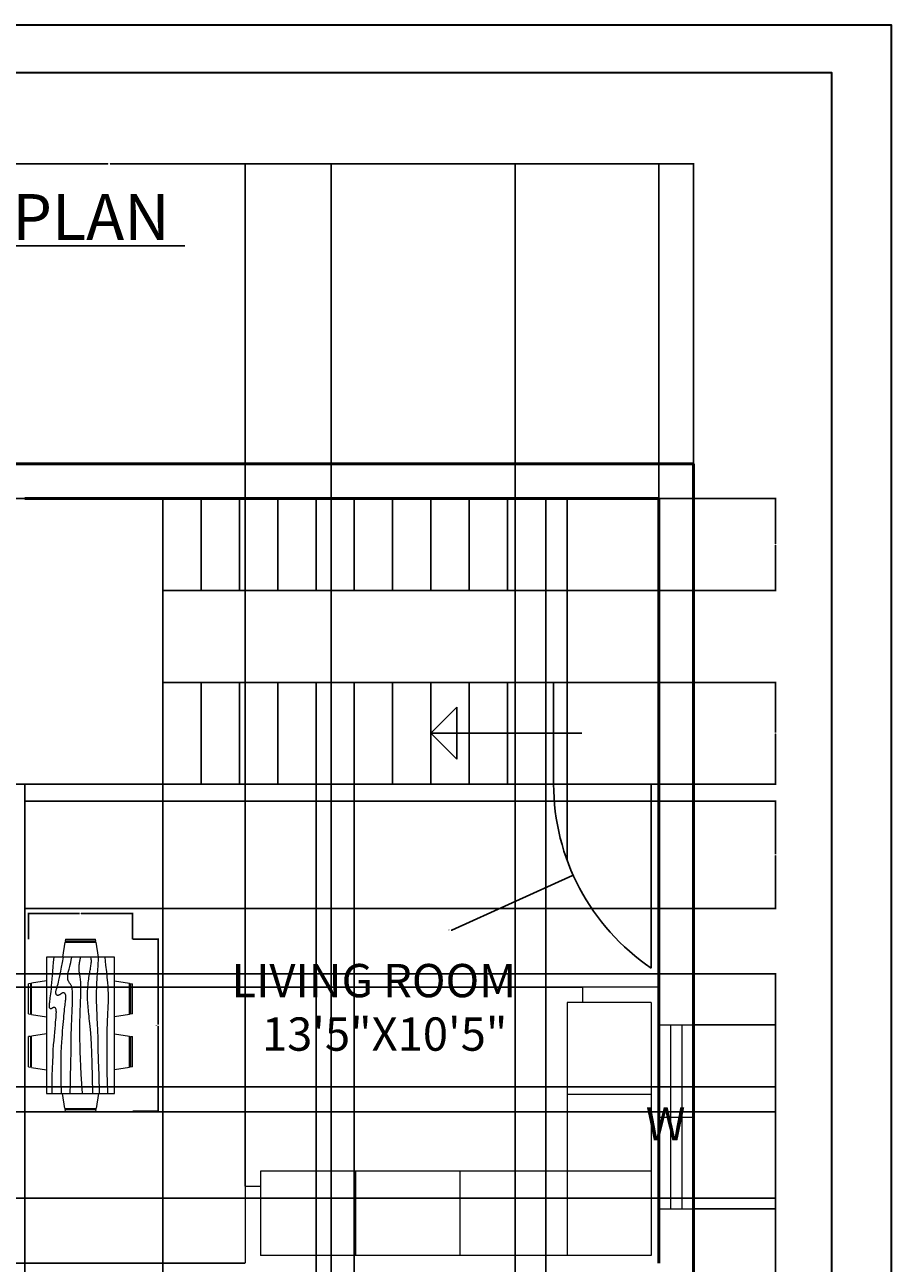
# Model space of a CAD drawing. Units: inches. Extents: x 1804 to 2221, y 1838 to 2403.
# Tile 3 of 3: x 1995 to 2221, y 2079 to 2403. Entities that reach past the tile are written whole.
import ezdxf

# ---------------------------------------------------------------- set-up
doc = ezdxf.new("R2010")
doc.units = ezdxf.units.IN
for name, color, linetype, lineweight in [('A-ANNO-DIMS', 2, 'Continuous', 18), ('A-ANNO-TEXT', 7, 'Continuous', 25), ('A-ANNO-TTLB', 7, 'Continuous', 35), ('A-AREA-IDEN', 7, 'Continuous', 25), ('A-DOOR', 3, 'Continuous', 25), ('A-FLOR-STRS', 7, 'Continuous', 25), ('A-FURN', 8, 'Continuous', 18), ('A-GLAZ', 4, 'Continuous', 18), ('A-WALL', 7, 'Continuous', 50)]:
    doc.layers.add(name, color=color, linetype=linetype, lineweight=lineweight)
doc.styles.get("Standard").update_dxf_attribs({"font": 'arial.ttf'})
doc.dimstyles.get("Standard").update_dxf_attribs({"dimtxt": 0.18, "dimasz": 0.18, "dimexe": 0.18, "dimexo": 0.0625, "dimgap": 0.09, "dimtad": 0, "dimtih": 1, "dimtoh": 1, "dimdec": 4, "dimzin": 0, "dimdsep": 46, "dimtxsty": 'Standard', "dimcen": 0.09, "dimadec": 0, "dimazin": 0, "dimtfac": 1, "dimtdec": 4, "dimtofl": 0, "dimtmove": 0, "dimatfit": 3, "dimfxl": 1, "dimtolj": 1, "dimtzin": 0, "dimarcsym": 0})

# ---------------------------------------------------------------- blocks, each defined once
blk = doc.blocks.new('Dining Set - 36 x 72 in.')
for p, q in [((-22, 27.5), (-22.1562, 26.50042)), ((-5.8416, 26.5), (-22.1534, 26.5)), ((-22, 27.5), (-6, 27.5)), ((-5.8437, 26.49966), (-6, 27.5)), ((6, 27.5), (5.8438, 26.50042)), ((22.1584, 26.5), (5.8466, 26.5)), ((6, 27.5), (22, 27.5)), ((22.1563, 26.49966), (22, 27.5)), ((-22.2343, 26.00059), (-23.4847, 17.99762)), ((-22.2304, 26), (-5.7608, 26)), ((-4.5152, 17.99762), (-5.7655, 25.99926)), ((5.7657, 26.00059), (4.5153, 17.99762)), ((5.7696, 26), (22.2392, 26)), ((23.4848, 17.99762), (22.2345, 25.99926)), ((36, 18), (-36, 18)), ((-36, 18), (-36, -18)), ((36, -18), (36, 18)), ((-45.5, 8), (-44.5004, 8.15617)), ((-45.5, 8), (-45.5, -8)), ((-44.5, -8.15843), (-44.5, 8.15338)), ((-44.0006, 8.23428), (-35.9976, 9.48474)), ((-44, 8.23041), (-44, -8.23915)), ((44.0006, 8.23428), (35.9976, 9.48474)), ((44, 8.23041), (44, -8.23915)), ((44.5, -8.15843), (44.5, 8.15338)), ((45.5, 8), (44.5005, 8.15617)), ((45.5, 8), (45.5, -8)), ((-44.4997, -8.15631), (-45.5, -8)), ((-35.9976, -9.48476), (-43.9993, -8.2345)), ((35.9976, -9.48476), (43.9993, -8.2345)), ((44.4997, -8.15631), (45.5, -8)), ((-36, -18), (36, -18)), ((-22.2343, -26.0006), (-23.4847, -17.99762)), ((-4.5152, -17.99762), (-5.7655, -25.99928)), ((5.7657, -26.0006), (4.5153, -17.99762)), ((23.4848, -17.99762), (22.2345, -25.99928)), ((-22.2304, -26), (-5.7608, -26)), ((5.7696, -26), (22.2392, -26)), ((-22, -27.5), (-22.1562, -26.50044)), ((-5.8416, -26.5), (-22.1534, -26.5)), ((-22, -27.5), (-6, -27.5)), ((-5.8437, -26.49967), (-6, -27.5)), ((6, -27.5), (5.8438, -26.50044)), ((22.1584, -26.5), (5.8466, -26.5)), ((6, -27.5), (22, -27.5)), ((22.1563, -26.49967), (22, -27.5))]:
    blk.add_line(p, q)
for points in [[(-36, 15), (-31.1772, 14.97754), (-26.8079, 14.91406), (-22.8538, 14.81543), (-19.276, 14.6875), (-16.0362, 14.53613), (-13.0957, 14.36718), (-10.4159, 14.18652), (-7.9583, 14), (-5.6904, 13.81315), (-3.6035, 13.63021), (-1.6954, 13.45508), (0.0365, 13.29166), (1.5945, 13.14388), (2.9811, 13.01562), (4.1988, 12.9108), (5.25, 12.83333), (6.1393, 12.78613), (6.8802, 12.76823), (7.4883, 12.77767), (7.9792, 12.8125), (8.3685, 12.87077), (8.6719, 12.95052), (8.9049, 13.0498), (9.0833, 13.16666), (9.2205, 13.29899), (9.3216, 13.44401), (9.3895, 13.59879), (9.4271, 13.76041), (9.4373, 13.92594), (9.4232, 14.09245), (9.3875, 14.257), (9.3333, 14.41666), (9.2638, 14.56917), (9.1836, 14.71484), (9.0975, 14.85465), (9.0104, 14.98958), (8.9272, 15.1206), (8.8529, 15.2487), (8.7922, 15.37483), (8.75, 15.5), (8.7305, 15.62467), (8.7344, 15.74739), (8.7617, 15.86621), (8.8125, 15.97916), (8.8867, 16.08431), (8.9844, 16.17968), (9.1055, 16.26334), (9.25, 16.33333), (9.4189, 16.38802), (9.6172, 16.42708), (9.8506, 16.45052), (10.125, 16.45833), (10.4463, 16.45052), (10.8203, 16.42708), (11.2529, 16.38802), (11.75, 16.33333), (12.3184, 16.26318), (12.9694, 16.17838), (13.7151, 16.07991), (14.5677, 15.96875), (15.5395, 15.84586), (16.6426, 15.71224), (17.8893, 15.56884), (19.2917, 15.41666), (20.859, 15.25667), (22.5879, 15.08984), (24.4721, 14.91715), (26.5052, 14.73958), (28.6809, 14.5581), (30.9929, 14.3737), (33.4347, 14.18733), (36, 14)], [(-36, 10), (-28.9766, 10.14274), (-23.1725, 10.20442), (-18.4241, 10.19775), (-14.5677, 10.13541), (-11.4399, 10.03011), (-8.877, 9.89453), (-6.7154, 9.74137), (-4.7917, 9.58333), (-2.9698, 9.43082), (-1.2246, 9.28515), (0.4415, 9.14534), (2.026, 9.01041), (3.5266, 8.87939), (4.9408, 8.7513), (6.266, 8.62516), (7.5, 8.5), (8.6411, 8.37549), (9.6914, 8.2539), (10.6538, 8.13818), (11.5312, 8.03125), (12.3267, 7.93603), (13.043, 7.85547), (13.6831, 7.79248), (14.25, 7.75), (14.7471, 7.7303), (15.1797, 7.73307), (15.5537, 7.75732), (15.875, 7.80208), (16.1494, 7.86637), (16.3828, 7.94922), (16.5811, 8.04964), (16.75, 8.16666), (16.8944, 8.29915), (17.0143, 8.44531), (17.1089, 8.60319), (17.1771, 8.77083), (17.218, 8.94629), (17.2305, 9.1276), (17.2137, 9.31282), (17.1667, 9.5), (17.0895, 9.6875), (16.987, 9.875), (16.8649, 10.0625), (16.7292, 10.25), (16.5856, 10.4375), (16.4401, 10.625), (16.2985, 10.8125), (16.1667, 11), (16.05, 11.18733), (15.9518, 11.3737), (15.8752, 11.5581), (15.8229, 11.73958), (15.798, 11.91715), (15.8034, 12.08984), (15.842, 12.25667), (15.9167, 12.41666), (16.0295, 12.56836), (16.1784, 12.70833), (16.3605, 12.83268), (16.5729, 12.9375), (16.8127, 13.01888), (17.0768, 13.07291), (17.3625, 13.0957), (17.6667, 13.08333), (17.9894, 13.03312), (18.3418, 12.94726), (18.7382, 12.82918), (19.1927, 12.68229), (19.7195, 12.51001), (20.3327, 12.31575), (21.0465, 12.10294), (21.875, 11.875), (22.8357, 11.63354), (23.959, 11.37304), (25.2786, 11.08618), (26.8282, 10.76562), (28.6414, 10.40405), (30.752, 9.99414), (33.1936, 9.52856), (36, 9)], [(-36, 5.5), (-30.7157, 5.3348), (-26.069, 5.20963), (-21.9946, 5.11767), (-18.4271, 5.05208), (-15.3009, 5.00602), (-12.5508, 4.97265), (-10.1112, 4.94515), (-7.9167, 4.91666), (-5.909, 4.88167), (-4.0586, 4.83984), (-2.3429, 4.79215), (-0.7396, 4.73958), (0.7739, 4.6831), (2.22, 4.6237), (3.6213, 4.56233), (5, 4.5), (6.373, 4.43782), (7.7344, 4.3776), (9.0723, 4.32129), (10.375, 4.27083), (11.6309, 4.22819), (12.8281, 4.19531), (13.9551, 4.17415), (15, 4.16666), (15.954, 4.17448), (16.819, 4.19791), (17.6001, 4.23698), (18.3021, 4.29166), (18.9299, 4.36198), (19.4883, 4.44791), (19.9823, 4.54948), (20.4167, 4.66666), (20.7969, 4.79899), (21.1302, 4.94401), (21.4245, 5.09879), (21.6875, 5.26041), (21.9271, 5.42594), (22.1511, 5.59245), (22.3672, 5.757), (22.5834, 5.91666), (22.8065, 6.06868), (23.0404, 6.21093), (23.2879, 6.34147), (23.5521, 6.45833), (23.8358, 6.55957), (24.142, 6.64323), (24.4735, 6.70735), (24.8334, 6.75), (25.2235, 6.76969), (25.642, 6.76692), (26.0858, 6.74267), (26.5521, 6.69791), (27.0379, 6.63362), (27.5404, 6.55078), (28.0565, 6.45036), (28.5834, 6.33333), (29.1242, 6.19987), (29.7071, 6.04687), (30.3661, 5.87044), (31.1354, 5.66666), (32.0493, 5.43164), (33.142, 5.16146), (34.4475, 4.85221), (36, 4.5)], [(-36, -1), (-30.7915, -0.6591), (-26.0195, -0.38216), (-21.6519, -0.16284), (-17.6563, 0.00521), (-14.0005, 0.12833), (-10.6523, 0.21289), (-7.5796, 0.26522), (-4.75, 0.29166), (-2.134, 0.29793), (0.2878, 0.28711), (2.5317, 0.26163), (4.6146, 0.22396), (6.5529, 0.17651), (8.3633, 0.12174), (10.0623, 0.06209), (11.6667, 0), (13.1899, -0.06201), (14.6341, -0.1211), (15.9982, -0.17432), (17.2813, -0.21875), (18.4823, -0.25147), (19.6003, -0.26953), (20.6343, -0.27002), (21.5834, -0.25), (22.4481, -0.20768), (23.2357, -0.14584), (23.9549, -0.06836), (24.6146, 0.02083), (25.2235, 0.11784), (25.7904, 0.21875), (26.3241, 0.31966), (26.8334, 0.41666), (27.3265, 0.50618), (27.8099, 0.58593), (28.2894, 0.65397), (28.7709, 0.70833), (29.2601, 0.74707), (29.763, 0.76823), (30.2855, 0.76985), (30.8334, 0.75), (31.4088, 0.70784), (31.9994, 0.64713), (32.589, 0.57275), (33.1615, 0.48958), (33.7008, 0.4025), (34.1908, 0.3164), (34.6153, 0.23616), (34.9584, 0.16666), (35.2099, 0.11165), (35.3848, 0.07031), (35.504, 0.04069), (35.5886, 0.02083), (35.6594, 0.00879), (35.7377, 0.0026), (35.8442, 0.00032), (36, 0)], [(-36, -6.5), (-27.1843, -6.31267), (-20.084, -6.1263), (-14.469, -5.9419), (-10.1094, -5.76042), (-6.7752, -5.58285), (-4.2363, -5.41016), (-2.2629, -5.24333), (-0.625, -5.08334), (0.8708, -4.93099), (2.2715, -4.78646), (3.5872, -4.64974), (4.8281, -4.52084), (6.0046, -4.39974), (7.127, -4.28646), (8.2053, -4.18099), (9.25, -4.08334), (10.2705, -3.99382), (11.2734, -3.91407), (12.2647, -3.84603), (13.25, -3.79167), (14.2354, -3.75293), (15.2266, -3.73177), (16.2295, -3.73015), (17.25, -3.75), (18.2912, -3.79248), (19.3451, -3.85547), (20.4009, -3.93604), (21.4479, -4.03125), (22.4754, -4.13819), (23.4727, -4.25391), (24.4289, -4.37549), (25.3334, -4.5), (26.1785, -4.62492), (26.9694, -4.74935), (27.7145, -4.87281), (28.4219, -4.99479), (29.1, -5.11483), (29.7572, -5.23242), (30.4016, -5.34709), (31.0417, -5.45834), (31.6837, -5.56437), (32.3262, -5.65821), (32.9658, -5.73153), (33.599, -5.77604), (34.2224, -5.78345), (34.8327, -5.74545), (35.4264, -5.65373), (36, -5.5)], [(-36, -10), (-26.4022, -9.81299), (-18.4675, -9.62891), (-11.9839, -9.45069), (-6.7396, -9.28125), (-2.5226, -9.12354), (0.8789, -8.98047), (3.6769, -8.85498), (6.0833, -8.75), (8.2767, -8.66765), (10.3021, -8.60677), (12.1712, -8.56543), (13.8958, -8.54167), (15.4876, -8.53353), (16.9583, -8.53907), (18.3197, -8.55632), (19.5834, -8.58334), (20.7616, -8.61841), (21.8685, -8.66081), (22.9188, -8.71004), (23.9271, -8.76563), (24.9081, -8.82707), (25.8763, -8.89388), (26.8465, -8.96558), (27.8334, -9.04167), (28.8474, -9.12118), (29.8828, -9.20117), (30.93, -9.27824), (31.9792, -9.34896), (33.0205, -9.40991), (34.0443, -9.45768), (35.0407, -9.48885), (36, -9.5)], [(-36, -14.5), (-30.0881, -14.33513), (-25.0332, -14.21224), (-20.7312, -14.12647), (-17.0781, -14.07292), (-13.97, -14.04671), (-11.3027, -14.04297), (-8.9724, -14.05681), (-6.875, -14.08334), (-4.9224, -14.11833), (-3.0905, -14.16016), (-1.3709, -14.20785), (0.2448, -14.26042), (1.7647, -14.3169), (3.1973, -14.3763), (4.5507, -14.43767), (5.8333, -14.5), (7.0554, -14.5621), (8.235, -14.62175), (9.3922, -14.67652), (10.5469, -14.72396), (11.7192, -14.76164), (12.929, -14.78711), (14.1965, -14.79794), (15.5417, -14.79167), (16.9933, -14.76424), (18.6152, -14.70508), (20.4804, -14.60197), (22.6615, -14.44271), (25.2312, -14.21509), (28.2624, -13.9069), (31.8277, -13.50594), (36, -13)]]:
    blk.add_lwpolyline(points)
blk = doc.blocks.new('*D18')
at = {"layer": 'A-ANNO-DIMS', "color": 0, "lineweight": -2, "transparency": 16777216}
for p, q in [((2022.76, 2163.97), (2029.61, 2163.97)), ((2029.43, 2163.79), (2029.43, 2141.72)), ((2029.43, 2119.28), (2029.43, 2141.35)), ((2022.76, 2119.1), (2029.61, 2119.1))]:
    blk.add_line(p, q, dxfattribs=at)
at = {"layer": 'A-ANNO-DIMS', "color": 0, "transparency": 16777216}
for points in [[(2029.4, 2163.79), (2029.46, 2163.79), (2029.43, 2163.97)], [(2029.4, 2119.28), (2029.46, 2119.28), (2029.43, 2119.1)]]:
    blk.add_solid(points, dxfattribs=at)
at = {"layer": 'Defpoints', "color": 0, "transparency": 16777216}
for p in [(2022.7, 2163.97), (2029.43, 2163.97), (2022.7, 2119.1)]:
    blk.add_point(p, dxfattribs=at)
at = {"layer": 'A-ANNO-DIMS', "color": 0, "transparency": 16777216, "insert": (2029.43, 2141.53), "char_height": 0.18, "attachment_point": 5}
blk.add_mtext('\\A1;DINETTE 45', dxfattribs=at)
blk = doc.blocks.new('*D19')
at = {"layer": 'A-ANNO-DIMS', "color": 0, "lineweight": -2, "transparency": 16777216}
for p, q in [((1995.58, 2164.03), (1995.58, 2170.88)), ((1995.76, 2170.7), (2008.92, 2170.7)), ((2022.52, 2170.7), (2009.36, 2170.7)), ((2022.7, 2164.03), (2022.7, 2170.88))]:
    blk.add_line(p, q, dxfattribs=at)
at = {"layer": 'A-ANNO-DIMS', "color": 0, "transparency": 16777216}
for points in [[(1995.76, 2170.73), (1995.76, 2170.67), (1995.58, 2170.7)], [(2022.52, 2170.73), (2022.52, 2170.67), (2022.7, 2170.7)]]:
    blk.add_solid(points, dxfattribs=at)
at = {"layer": 'Defpoints', "color": 0, "transparency": 16777216}
for p in [(1995.58, 2170.7), (1995.58, 2163.97), (2022.7, 2163.97)]:
    blk.add_point(p, dxfattribs=at)
at = {"layer": 'A-ANNO-DIMS', "color": 0, "transparency": 16777216, "insert": (2009.14, 2170.7), "char_height": 0.18, "attachment_point": 5}
blk.add_mtext('\\A1;27', dxfattribs=at)
blk = doc.blocks.new('*D32')
at = {"layer": 'A-ANNO-DIMS', "color": 0, "lineweight": -2, "transparency": 16777216}
for p, q in [((1864.1, 2288.03), (1864.1, 2366.45)), ((1864.28, 2366.27), (2016.31, 2366.27)), ((2168.92, 2366.27), (2016.89, 2366.27)), ((2169.1, 2288.03), (2169.1, 2366.45))]:
    blk.add_line(p, q, dxfattribs=at)
at = {"layer": 'A-ANNO-DIMS', "color": 0, "transparency": 16777216}
for points in [[(1864.28, 2366.3), (1864.28, 2366.24), (1864.1, 2366.27)], [(2168.92, 2366.3), (2168.92, 2366.24), (2169.1, 2366.27)]]:
    blk.add_solid(points, dxfattribs=at)
at = {"layer": 'Defpoints', "color": 0, "transparency": 16777216}
for p in [(2169.1, 2366.27), (1864.1, 2287.97), (2169.1, 2287.97)]:
    blk.add_point(p, dxfattribs=at)
at = {"layer": 'A-ANNO-DIMS', "color": 0, "transparency": 16777216, "insert": (2016.6, 2366.27), "char_height": 0.18, "attachment_point": 5}
blk.add_mtext('\\A1;305', dxfattribs=at)
blk = doc.blocks.new('*D37')
at = {"layer": 'A-ANNO-DIMS', "color": 0, "lineweight": -2, "transparency": 16777216}
for p, q in [((2169.16, 2093.67), (2190.68, 2093.67)), ((2190.5, 2093.49), (2190.5, 2026.5)), ((2190.5, 1959.15), (2190.5, 2026.14)), ((2169.16, 1958.97), (2190.68, 1958.97))]:
    blk.add_line(p, q, dxfattribs=at)
at = {"layer": 'A-ANNO-DIMS', "color": 0, "transparency": 16777216}
for points in [[(2190.47, 2093.49), (2190.53, 2093.49), (2190.5, 2093.67)], [(2190.47, 1959.15), (2190.53, 1959.15), (2190.5, 1958.97)]]:
    blk.add_solid(points, dxfattribs=at)
at = {"layer": 'Defpoints', "color": 0, "transparency": 16777216}
for p in [(2169.1, 2093.67), (2190.5, 2093.67), (2169.1, 1958.97)]:
    blk.add_point(p, dxfattribs=at)
at = {"layer": 'A-ANNO-DIMS', "color": 0, "transparency": 16777216, "insert": (2190.5, 2026.32), "char_height": 0.18, "attachment_point": 5}
blk.add_mtext('\\A1;134.7', dxfattribs=at)
blk = doc.blocks.new('*D38')
at = {"layer": 'A-ANNO-DIMS', "color": 0, "lineweight": -2, "transparency": 16777216}
for p, q in [((2169.16, 2141.67), (2190.68, 2141.67)), ((2190.5, 2141.49), (2190.5, 2117.85)), ((2190.5, 2093.85), (2190.5, 2117.49)), ((2169.16, 2093.67), (2190.68, 2093.67))]:
    blk.add_line(p, q, dxfattribs=at)
at = {"layer": 'A-ANNO-DIMS', "color": 0, "transparency": 16777216}
for points in [[(2190.47, 2141.49), (2190.53, 2141.49), (2190.5, 2141.67)], [(2190.47, 2093.85), (2190.53, 2093.85), (2190.5, 2093.67)]]:
    blk.add_solid(points, dxfattribs=at)
at = {"layer": 'Defpoints', "color": 0, "transparency": 16777216}
for p in [(2169.1, 2141.67), (2190.5, 2141.67), (2169.1, 2093.67)]:
    blk.add_point(p, dxfattribs=at)
at = {"layer": 'A-ANNO-DIMS', "color": 0, "transparency": 16777216, "insert": (2190.5, 2117.67), "char_height": 0.18, "attachment_point": 5}
blk.add_mtext('\\A1;48', dxfattribs=at)
blk = doc.blocks.new('*D41')
at = {"layer": 'A-ANNO-DIMS', "color": 0, "lineweight": -2, "transparency": 16777216}
for p, q in [((1994.6, 2204.41), (1994.6, 1937.39)), ((2030.6, 2204.41), (2030.6, 1937.39)), ((1994.78, 1937.57), (2012.38, 1937.57)), ((2030.42, 1937.57), (2012.82, 1937.57))]:
    blk.add_line(p, q, dxfattribs=at)
at = {"layer": 'A-ANNO-DIMS', "color": 0, "transparency": 16777216}
for points in [[(1994.78, 1937.6), (1994.78, 1937.54), (1994.6, 1937.57)], [(2030.42, 1937.6), (2030.42, 1937.54), (2030.6, 1937.57)]]:
    blk.add_solid(points, dxfattribs=at)
at = {"layer": 'Defpoints', "color": 0, "transparency": 16777216}
for p in [(1994.6, 2204.47), (2030.6, 2204.47), (2030.6, 1937.57)]:
    blk.add_point(p, dxfattribs=at)
at = {"layer": 'A-ANNO-DIMS', "color": 0, "transparency": 16777216, "insert": (2012.6, 1937.57), "char_height": 0.18, "attachment_point": 5}
blk.add_mtext('\\A1;36', dxfattribs=at)
blk = doc.blocks.new('*D42')
at = {"layer": 'A-ANNO-DIMS', "color": 0, "lineweight": -2, "transparency": 16777216}
for p, q in [((2030.6, 2254.91), (2030.6, 1937.39)), ((2130.6, 2254.91), (2130.6, 1937.39)), ((2030.78, 1937.57), (2080.32, 1937.57)), ((2130.42, 1937.57), (2080.88, 1937.57))]:
    blk.add_line(p, q, dxfattribs=at)
at = {"layer": 'A-ANNO-DIMS', "color": 0, "transparency": 16777216}
for points in [[(2030.78, 1937.6), (2030.78, 1937.54), (2030.6, 1937.57)], [(2130.42, 1937.6), (2130.42, 1937.54), (2130.6, 1937.57)]]:
    blk.add_solid(points, dxfattribs=at)
at = {"layer": 'Defpoints', "color": 0, "transparency": 16777216}
for p in [(2030.6, 2254.97), (2130.6, 2254.97), (2130.6, 1937.57)]:
    blk.add_point(p, dxfattribs=at)
at = {"layer": 'A-ANNO-DIMS', "color": 0, "transparency": 16777216, "insert": (2080.6, 1937.57), "char_height": 0.18, "attachment_point": 5}
blk.add_mtext('\\A1;100', dxfattribs=at)
blk = doc.blocks.new('*D43')
at = {"layer": 'A-ANNO-DIMS', "color": 0, "lineweight": -2, "transparency": 16777216}
for p, q in [((2030.54, 2278.97), (1842.52, 2278.97)), ((1842.7, 2278.79), (1842.7, 2241.9)), ((1842.7, 2204.65), (1842.7, 2241.54)), ((2030.54, 2204.47), (1842.52, 2204.47))]:
    blk.add_line(p, q, dxfattribs=at)
at = {"layer": 'A-ANNO-DIMS', "color": 0, "transparency": 16777216}
for points in [[(1842.67, 2278.79), (1842.73, 2278.79), (1842.7, 2278.97)], [(1842.67, 2204.65), (1842.73, 2204.65), (1842.7, 2204.47)]]:
    blk.add_solid(points, dxfattribs=at)
at = {"layer": 'Defpoints', "color": 0, "transparency": 16777216}
for p in [(1842.7, 2278.97), (2030.6, 2278.97), (2030.6, 2204.47)]:
    blk.add_point(p, dxfattribs=at)
at = {"layer": 'A-ANNO-DIMS', "color": 0, "transparency": 16777216, "insert": (1842.7, 2241.72), "char_height": 0.18, "attachment_point": 5}
blk.add_mtext('\\A1;74.5', dxfattribs=at)
blk = doc.blocks.new('*D44')
at = {"layer": 'A-ANNO-DIMS', "color": 0, "lineweight": -2, "transparency": 16777216}
for p, q in [((2070.6, 2204.41), (2070.6, 1937.39)), ((2080.6, 2204.41), (2080.6, 1937.39)), ((2070.78, 1937.57), (2075.39, 1937.57)), ((2080.42, 1937.57), (2075.81, 1937.57))]:
    blk.add_line(p, q, dxfattribs=at)
at = {"layer": 'A-ANNO-DIMS', "color": 0, "transparency": 16777216}
for points in [[(2070.78, 1937.6), (2070.78, 1937.54), (2070.6, 1937.57)], [(2080.42, 1937.6), (2080.42, 1937.54), (2080.6, 1937.57)]]:
    blk.add_solid(points, dxfattribs=at)
at = {"layer": 'Defpoints', "color": 0, "transparency": 16777216}
for p in [(2070.6, 2204.47), (2080.6, 2204.47), (2080.6, 1937.57)]:
    blk.add_point(p, dxfattribs=at)
at = {"layer": 'A-ANNO-DIMS', "color": 0, "transparency": 16777216, "insert": (2075.6, 1937.57), "char_height": 0.18, "attachment_point": 5}
blk.add_mtext('\\A1;10', dxfattribs=at)
blk = doc.blocks.new('*D45')
at = {"layer": 'A-ANNO-DIMS', "color": 0, "lineweight": -2, "transparency": 16777216}
for p, q in [((2130.66, 2278.97), (2190.68, 2278.97)), ((2190.5, 2278.79), (2190.5, 2267.15)), ((2190.5, 2255.15), (2190.5, 2266.79)), ((2130.66, 2254.97), (2190.68, 2254.97))]:
    blk.add_line(p, q, dxfattribs=at)
at = {"layer": 'A-ANNO-DIMS', "color": 0, "transparency": 16777216}
for points in [[(2190.47, 2278.79), (2190.53, 2278.79), (2190.5, 2278.97)], [(2190.47, 2255.15), (2190.53, 2255.15), (2190.5, 2254.97)]]:
    blk.add_solid(points, dxfattribs=at)
at = {"layer": 'Defpoints', "color": 0, "transparency": 16777216}
for p in [(2130.6, 2278.97), (2190.5, 2278.97), (2130.6, 2254.97)]:
    blk.add_point(p, dxfattribs=at)
at = {"layer": 'A-ANNO-DIMS', "color": 0, "transparency": 16777216, "insert": (2190.5, 2266.97), "char_height": 0.18, "attachment_point": 5}
blk.add_mtext('\\A1;24', dxfattribs=at)
blk = doc.blocks.new('*D46')
at = {"layer": 'A-ANNO-DIMS', "color": 0, "lineweight": -2, "transparency": 16777216}
for p, q in [((2132.66, 2230.97), (2190.68, 2230.97)), ((2190.5, 2230.79), (2190.5, 2217.9)), ((2190.5, 2204.65), (2190.5, 2217.54)), ((2132.66, 2204.47), (2190.68, 2204.47))]:
    blk.add_line(p, q, dxfattribs=at)
at = {"layer": 'A-ANNO-DIMS', "color": 0, "transparency": 16777216}
for points in [[(2190.47, 2230.79), (2190.53, 2230.79), (2190.5, 2230.97)], [(2190.47, 2204.65), (2190.53, 2204.65), (2190.5, 2204.47)]]:
    blk.add_solid(points, dxfattribs=at)
at = {"layer": 'Defpoints', "color": 0, "transparency": 16777216}
for p in [(2132.6, 2230.97), (2190.5, 2230.97), (2132.6, 2204.47)]:
    blk.add_point(p, dxfattribs=at)
at = {"layer": 'A-ANNO-DIMS', "color": 0, "transparency": 16777216, "insert": (2190.5, 2217.72), "char_height": 0.18, "attachment_point": 5}
blk.add_mtext('\\A1;26.5', dxfattribs=at)
blk = doc.blocks.new('*D47')
at = {"layer": 'A-ANNO-DIMS', "color": 0, "lineweight": -2, "transparency": 16777216}
for p, q in [((2052.1, 2099.53), (2052.1, 2366.45)), ((2052.28, 2366.27), (2105.82, 2366.27)), ((2159.92, 2366.27), (2106.38, 2366.27)), ((2160.1, 2151.53), (2160.1, 2366.45))]:
    blk.add_line(p, q, dxfattribs=at)
at = {"layer": 'A-ANNO-DIMS', "color": 0, "transparency": 16777216}
for points in [[(2052.28, 2366.3), (2052.28, 2366.24), (2052.1, 2366.27)], [(2159.92, 2366.3), (2159.92, 2366.24), (2160.1, 2366.27)]]:
    blk.add_solid(points, dxfattribs=at)
at = {"layer": 'Defpoints', "color": 0, "transparency": 16777216}
for p in [(2160.1, 2366.27), (2160.1, 2151.47), (2052.1, 2099.47)]:
    blk.add_point(p, dxfattribs=at)
at = {"layer": 'A-ANNO-DIMS', "color": 0, "transparency": 16777216, "insert": (2106.1, 2366.27), "char_height": 0.18, "attachment_point": 5}
blk.add_mtext('\\A1;108', dxfattribs=at)
blk = doc.blocks.new('*D48')
at = {"layer": 'A-ANNO-DIMS', "color": 0, "lineweight": -2, "transparency": 16777216}
for p, q in [((2140.04, 2151.47), (1842.52, 2151.47)), ((1842.7, 2151.29), (1842.7, 2115.65)), ((1842.7, 2079.65), (1842.7, 2115.29)), ((2052.04, 2079.47), (1842.52, 2079.47))]:
    blk.add_line(p, q, dxfattribs=at)
at = {"layer": 'A-ANNO-DIMS', "color": 0, "transparency": 16777216}
for points in [[(1842.67, 2151.29), (1842.73, 2151.29), (1842.7, 2151.47)], [(1842.67, 2079.65), (1842.73, 2079.65), (1842.7, 2079.47)]]:
    blk.add_solid(points, dxfattribs=at)
at = {"layer": 'Defpoints', "color": 0, "transparency": 16777216}
for p in [(1842.7, 2151.47), (2140.1, 2151.47), (2052.1, 2079.47)]:
    blk.add_point(p, dxfattribs=at)
at = {"layer": 'A-ANNO-DIMS', "color": 0, "transparency": 16777216, "insert": (1842.7, 2115.47), "char_height": 0.18, "attachment_point": 5}
blk.add_mtext('\\A1;72', dxfattribs=at)
blk = doc.blocks.new('*D49')
at = {"layer": 'A-ANNO-DIMS', "color": 0, "lineweight": -2, "transparency": 16777216}
for p, q in [((1994.66, 2199.97), (2190.68, 2199.97)), ((2190.5, 2199.79), (2190.5, 2186.15)), ((2190.5, 2172.15), (2190.5, 2185.79)), ((1994.66, 2171.97), (2190.68, 2171.97))]:
    blk.add_line(p, q, dxfattribs=at)
at = {"layer": 'A-ANNO-DIMS', "color": 0, "transparency": 16777216}
for points in [[(2190.47, 2199.79), (2190.53, 2199.79), (2190.5, 2199.97)], [(2190.47, 2172.15), (2190.53, 2172.15), (2190.5, 2171.97)]]:
    blk.add_solid(points, dxfattribs=at)
at = {"layer": 'Defpoints', "color": 0, "transparency": 16777216}
for p in [(1994.6, 2199.97), (2190.5, 2199.97), (1994.6, 2171.97)]:
    blk.add_point(p, dxfattribs=at)
at = {"layer": 'A-ANNO-DIMS', "color": 0, "transparency": 16777216, "insert": (2190.5, 2185.97), "char_height": 0.18, "attachment_point": 5}
blk.add_mtext('\\A1;28', dxfattribs=at)
blk = doc.blocks.new('*D51')
at = {"layer": 'A-ANNO-DIMS', "color": 0, "lineweight": -2, "transparency": 16777216}
for p, q in [((1913.16, 2118.97), (2190.68, 2118.97)), ((2190.5, 2118.79), (2190.5, 2107.9)), ((2190.5, 2096.65), (2190.5, 2107.54)), ((1913.16, 2096.47), (2190.68, 2096.47))]:
    blk.add_line(p, q, dxfattribs=at)
at = {"layer": 'A-ANNO-DIMS', "color": 0, "transparency": 16777216}
for points in [[(2190.47, 2118.79), (2190.53, 2118.79), (2190.5, 2118.97)], [(2190.47, 2096.65), (2190.53, 2096.65), (2190.5, 2096.47)]]:
    blk.add_solid(points, dxfattribs=at)
at = {"layer": 'Defpoints', "color": 0, "transparency": 16777216}
for p in [(1913.1, 2118.97), (2190.5, 2118.97), (1913.1, 2096.47)]:
    blk.add_point(p, dxfattribs=at)
at = {"layer": 'A-ANNO-DIMS', "color": 0, "transparency": 16777216, "insert": (2190.5, 2107.72), "char_height": 0.18, "attachment_point": 5}
blk.add_mtext('\\A1;22.5', dxfattribs=at)
blk = doc.blocks.new('*D52')
at = {"layer": 'A-ANNO-DIMS', "color": 0, "lineweight": -2, "transparency": 16777216}
for p, q in [((1966.16, 2154.97), (2190.68, 2154.97)), ((2190.5, 2154.79), (2190.5, 2140.4)), ((2190.5, 2125.65), (2190.5, 2140.04)), ((1966.16, 2125.47), (2190.68, 2125.47))]:
    blk.add_line(p, q, dxfattribs=at)
at = {"layer": 'A-ANNO-DIMS', "color": 0, "transparency": 16777216}
for points in [[(2190.47, 2154.79), (2190.53, 2154.79), (2190.5, 2154.97)], [(2190.47, 2125.65), (2190.53, 2125.65), (2190.5, 2125.47)]]:
    blk.add_solid(points, dxfattribs=at)
at = {"layer": 'Defpoints', "color": 0, "transparency": 16777216}
for p in [(1966.1, 2154.97), (2190.5, 2154.97), (1966.1, 2125.47)]:
    blk.add_point(p, dxfattribs=at)
at = {"layer": 'A-ANNO-DIMS', "color": 0, "transparency": 16777216, "insert": (2190.5, 2140.22), "char_height": 0.18, "attachment_point": 5}
blk.add_mtext('\\A1;29.5', dxfattribs=at)
blk = doc.blocks.new('*D54')
at = {"layer": 'A-ANNO-DIMS', "color": 0, "lineweight": -2, "transparency": 16777216}
for p, q in [((2074.6, 2075.03), (2074.6, 2366.45)), ((2074.78, 2366.27), (2098.38, 2366.27)), ((2122.42, 2366.27), (2098.82, 2366.27)), ((2122.6, 2075.03), (2122.6, 2366.45))]:
    blk.add_line(p, q, dxfattribs=at)
at = {"layer": 'A-ANNO-DIMS', "color": 0, "transparency": 16777216}
for points in [[(2074.78, 2366.3), (2074.78, 2366.24), (2074.6, 2366.27)], [(2122.42, 2366.3), (2122.42, 2366.24), (2122.6, 2366.27)]]:
    blk.add_solid(points, dxfattribs=at)
at = {"layer": 'Defpoints', "color": 0, "transparency": 16777216}
for p in [(2122.6, 2366.27), (2074.6, 2074.97), (2122.6, 2074.97)]:
    blk.add_point(p, dxfattribs=at)
at = {"layer": 'A-ANNO-DIMS', "color": 0, "transparency": 16777216, "insert": (2098.6, 2366.27), "char_height": 0.18, "attachment_point": 5}
blk.add_mtext('\\A1;48', dxfattribs=at)
blk = doc.blocks.new('*D60')
at = {"layer": 'A-ANNO-DIMS', "color": 0, "lineweight": -2, "transparency": 16777216}
for p, q in [((1949.97, 2221.04), (1950.15, 2221.04)), ((1950.15, 2221.04), (1966.73, 2192.61)), ((1994.51, 2144.83), (1994.69, 2144.83)), ((1994.6, 2144.74), (1994.6, 2144.92))]:
    blk.add_line(p, q, dxfattribs=at)
at = {"layer": 'A-ANNO-DIMS', "color": 0, "transparency": 16777216}
blk.add_solid([(1966.75, 2192.63), (1966.7, 2192.6), (1966.82, 2192.46)], dxfattribs=at)
at = {"layer": 'Defpoints', "color": 0, "transparency": 16777216}
for p in [(1966.82, 2192.46), (1994.6, 2144.83)]:
    blk.add_point(p, dxfattribs=at)
at = {"layer": 'A-ANNO-DIMS', "color": 0, "transparency": 16777216, "insert": (1949.49, 2221.04), "char_height": 0.18, "attachment_point": 5}
blk.add_mtext('\\A1;R55.14', dxfattribs=at)
blk = doc.blocks.new('*D61')
at = {"layer": 'A-ANNO-DIMS', "color": 0, "lineweight": -2, "transparency": 16777216}
for p, q in [((2005.51, 2079.47), (2005.69, 2079.47)), ((2005.6, 2079.38), (2005.6, 2079.56)), ((2053.12, 2031.95), (2035.43, 2049.64)), ((2053.3, 2031.95), (2053.12, 2031.95))]:
    blk.add_line(p, q, dxfattribs=at)
at = {"layer": 'A-ANNO-DIMS', "color": 0, "transparency": 16777216}
blk.add_solid([(2035.45, 2049.66), (2035.41, 2049.62), (2035.3, 2049.77)], dxfattribs=at)
at = {"layer": 'Defpoints', "color": 0, "transparency": 16777216}
for p in [(2005.6, 2079.47), (2035.3, 2049.77)]:
    blk.add_point(p, dxfattribs=at)
at = {"layer": 'A-ANNO-DIMS', "color": 0, "transparency": 16777216, "insert": (2053.6, 2031.95), "char_height": 0.18, "attachment_point": 5}
blk.add_mtext('\\A1;R42', dxfattribs=at)
blk = doc.blocks.new('*D65')
at = {"layer": 'A-ANNO-DIMS', "color": 0, "lineweight": -2, "transparency": 16777216}
for p, q in [((2190.44, 2204.47), (2190.62, 2204.47)), ((2190.53, 2204.38), (2190.53, 2204.56)), ((2106.04, 2166.37), (2137.56, 2180.58)), ((2105.86, 2166.37), (2106.04, 2166.37))]:
    blk.add_line(p, q, dxfattribs=at)
at = {"layer": 'A-ANNO-DIMS', "color": 0, "transparency": 16777216}
blk.add_solid([(2137.54, 2180.61), (2137.57, 2180.56), (2137.72, 2180.66)], dxfattribs=at)
at = {"layer": 'Defpoints', "color": 0, "transparency": 16777216}
for p in [(2190.53, 2204.47), (2137.72, 2180.66)]:
    blk.add_point(p, dxfattribs=at)
at = {"layer": 'A-ANNO-DIMS', "color": 0, "transparency": 16777216, "insert": (2105.38, 2166.37), "char_height": 0.18, "attachment_point": 5}
blk.add_mtext('\\A1;R57.93', dxfattribs=at)

msp = doc.modelspace()

# ---------------------------------------------------------------- linework, layer by layer
at = {"layer": 'A-ANNO-TEXT'}
msp.add_line((1989.0457, 2344.8659), (2036.3709, 2344.8659), dxfattribs=at)
at = {"layer": 'A-ANNO-TTLB'}
for points in [[(1804.4104, 2402.5437), (2220.7086, 2402.5437), (2220.7086, 1837.8762), (1804.4104, 1837.8762)], [(1817.9401, 2390.0649), (2205.0975, 2390.0649), (2205.0975, 1852.4349), (1817.9401, 1852.4349)]]:
    msp.add_lwpolyline(points, close=True, dxfattribs=at)
at = {"layer": 'A-DOOR'}
for q in [(2158.1006, 2156.4683), (2160.1006, 2204.4683)]:
    msp.add_line((2158.1006, 2204.4683), q, dxfattribs=at)
msp.add_arc((2190.5271, 2204.4683), 57.9265, 180, 235.958949, dxfattribs=at)
at = {"layer": 'A-FLOR-STRS'}
for p, q in [((2030.6006, 2278.9683), (2030.6006, 2204.4683)), ((2040.6006, 2278.9683), (2040.6006, 2254.9683)), ((2050.6006, 2278.9683), (2050.6006, 2254.9683)), ((2060.6006, 2278.9683), (2060.6006, 2254.9683)), ((2070.6006, 2278.9683), (2070.6006, 2254.9683)), ((2080.6006, 2278.9683), (2080.6006, 2254.9683)), ((2090.6006, 2278.9683), (2090.6006, 2254.9683)), ((2100.6006, 2278.9683), (2100.6006, 2254.9683)), ((2110.6006, 2278.9683), (2110.6006, 2254.9683)), ((2120.6006, 2278.9683), (2120.6006, 2254.9683)), ((2130.6006, 2278.9683), (2130.6006, 2204.4683)), ((2136.1006, 2278.9683), (2136.1006, 2184.6381)), ((2030.6006, 2254.9683), (2130.6006, 2254.9683)), ((2030.6006, 2230.9683), (2132.6006, 2230.9683)), ((2040.6006, 2230.9683), (2040.6006, 2204.4683)), ((2050.6006, 2230.9683), (2050.6006, 2204.4683)), ((2060.6006, 2230.9683), (2060.6006, 2204.4683)), ((2070.6006, 2230.9683), (2070.6006, 2204.4683)), ((2080.6006, 2230.9683), (2080.6006, 2204.4683)), ((2090.6006, 2230.9683), (2090.6006, 2204.4683)), ((2100.6006, 2230.9683), (2100.6006, 2204.4683)), ((2110.6006, 2230.9683), (2110.6006, 2204.4683)), ((2120.6006, 2230.9683), (2120.6006, 2204.4683)), ((2132.6006, 2230.9683), (2132.6006, 2204.4683)), ((2100.6006, 2217.7183), (2107.3911, 2224.4869)), ((2107.3911, 2224.4869), (2107.3911, 2210.9497)), ((2100.6006, 2217.7183), (2139.9499, 2217.7183)), ((2100.6006, 2217.7183), (2107.3911, 2210.9497)), ((1994.6006, 2204.4683), (2132.6006, 2204.4683))]:
    msp.add_line(p, q, dxfattribs=at)
at = {"layer": 'A-FURN'}
for p, q in [((2160.1006, 2151.4683), (2140.1006, 2151.4683)), ((2140.1006, 2151.4683), (2140.1006, 2147.4683)), ((2136.1006, 2147.4683), (2136.1006, 2081.4683)), ((2158.1006, 2147.4683), (2136.1006, 2147.4683)), ((2158.1006, 2147.4683), (2158.1006, 2081.4683)), ((2158.1006, 2123.4683), (2136.1006, 2123.4683)), ((2158.1006, 2103.4683), (2056.1006, 2103.4683)), ((2056.1006, 2103.4683), (2056.1006, 2081.4683)), ((2080.8674, 2103.4683), (2080.8674, 2081.4683)), ((2108.1006, 2103.4683), (2108.1006, 2081.4683)), ((2052.1006, 2099.4683), (2052.1006, 2079.4683)), ((2056.1006, 2099.4683), (2052.1006, 2099.4683)), ((2158.1006, 2081.4683), (2056.1006, 2081.4683))]:
    msp.add_line(p, q, dxfattribs=at)
at = {"layer": 'A-GLAZ'}
for p, q in [((2160.1006, 2141.6724), (2169.1006, 2141.6724)), ((2163.1006, 2141.6724), (2163.1006, 2093.6724)), ((2166.1006, 2141.6724), (2166.1006, 2093.6724)), ((2160.1006, 2117.5811), (2169.1006, 2117.5811)), ((2160.1006, 2093.6724), (2169.1006, 2093.6724))]:
    msp.add_line(p, q, dxfattribs=at)
at = {"layer": 'A-WALL'}
for p, q in [((1864.1006, 2287.9683), (2169.1006, 2287.9683)), ((2169.1006, 2287.9683), (2169.1006, 1958.9683)), ((1994.6006, 2278.9683), (2160.1006, 2278.9683)), ((2160.1006, 2278.9683), (2160.1006, 2079.4683))]:
    msp.add_line(p, q, dxfattribs=at)

# ---------------------------------------------------------------- block references
at = {"layer": 'A-FURN', "xscale": 0.493100188170388, "yscale": 0.493100188170388, "zscale": 0.493100188170388, "rotation": 89.99999999999996}
msp.add_blockref('Dining Set - 36 x 72 in.', (2009.1376, 2141.5349), dxfattribs=at)

# ---------------------------------------------------------------- texts
at = {"layer": 'A-ANNO-TEXT'}
for s, height, p in [('PLAN', 12, (1991.349, 2346.384)), ('                     W', 8.682741, (2100.9001, 2111.4938))]:
    msp.add_text(s, height=height, dxfattribs=at).set_placement(p)
at = {"layer": 'A-AREA-IDEN'}
for s, p in [('LIVING ROOM', (2048.5311, 2148.8584)), ('   13\'5"X10\'5"', (2048.5311, 2134.9103))]:
    msp.add_text(s, height=8.682741, dxfattribs=at).set_placement(p)

# ---------------------------------------------------------------- dimensions: what is measured, and where the dimension line sits
at = {"layer": 'A-ANNO-DIMS'}
for base, p1, p2, picture, middle in [((2169.1006, 2366.2659), (1864.1006, 2287.9683), (2169.1006, 2287.9683), '*D32', (2016.6006, 2366.2659)), ((2160.1006, 2366.2659), (2052.1006, 2099.4683), (2160.1006, 2151.4683), '*D47', (2106.1006, 2366.2659)), ((2122.6006, 2366.2659), (2074.6006, 2074.9683), (2122.6006, 2074.9683), '*D54', (2098.6006, 2366.2659)), ((2130.6006, 1937.5683), (2030.6006, 2254.9683), (2130.6006, 2254.9683), '*D42', (2080.6006, 1937.5683)), ((2030.6006, 1937.5683), (1994.6006, 2204.4683), (2030.6006, 2204.4683), '*D41', (2012.6006, 1937.5683)), ((2080.6006, 1937.5683), (2070.6006, 2204.4683), (2080.6006, 2204.4683), '*D44', (2075.6006, 1937.5683))]:
    dim = msp.add_linear_dim(base=base, p1=p1, p2=p2, dimstyle='Standard', override={"dimdec": 0, "dimlfac": 1, "dimrnd": 0, "dimzin": 0, "dimdsep": 46, "dimlunit": 2}, dxfattribs=at)
    dim.commit()
    dim.dimension.update_dxf_attribs({"geometry": picture, "text_midpoint": middle})
for base, p1, p2, angle, override, picture, middle in [((1842.7006, 2278.9683), (2030.6006, 2204.4683), (2030.6006, 2278.9683), 90, {"dimdec": 1, "dimlfac": 1, "dimrnd": 0, "dimzin": 0, "dimdsep": 46, "dimlunit": 2}, '*D43', (1842.7006, 2241.7183)), ((2190.5006, 2278.9683), (2130.6006, 2254.9683), (2130.6006, 2278.9683), 90, {"dimdec": 0, "dimlfac": 1, "dimrnd": 0, "dimzin": 0, "dimdsep": 46, "dimlunit": 2}, '*D45', (2190.5006, 2266.9683)), ((2190.5006, 2230.9683), (2132.6006, 2204.4683), (2132.6006, 2230.9683), 90, {"dimdec": 1, "dimlfac": 1, "dimrnd": 0, "dimzin": 0, "dimdsep": 46, "dimlunit": 2}, '*D46', (2190.5006, 2217.7183)), ((2190.5006, 2199.9683), (1994.6006, 2171.9683), (1994.6006, 2199.9683), 90, {"dimdec": 0, "dimlfac": 1, "dimrnd": 0, "dimzin": 0, "dimdsep": 46, "dimlunit": 2}, '*D49', (2190.5006, 2185.9683)), ((1995.5773, 2170.7018), (2022.6978, 2163.971), (1995.5773, 2163.971), 180, {"dimdec": 0, "dimlfac": 1, "dimrnd": 0, "dimzin": 0, "dimdsep": 46, "dimlunit": 2}, '*D19', (2009.1376, 2170.7018)), ((2190.5006, 2154.9683), (1966.1006, 2125.4683), (1966.1006, 2154.9683), 90, {"dimdec": 1, "dimlfac": 1, "dimrnd": 0, "dimzin": 0, "dimdsep": 46, "dimlunit": 2}, '*D52', (2190.5006, 2140.2183)), ((1842.7006, 2151.4683), (2052.1006, 2079.4683), (2140.1006, 2151.4683), 90, {"dimdec": 0, "dimlfac": 1, "dimrnd": 0, "dimzin": 0, "dimdsep": 46, "dimlunit": 2}, '*D48', (1842.7006, 2115.4683)), ((2190.5006, 2141.6724), (2169.1006, 2093.6724), (2169.1006, 2141.6724), 90, {"dimdec": 0, "dimlfac": 1, "dimrnd": 0, "dimzin": 0, "dimdsep": 46, "dimlunit": 2}, '*D38', (2190.5006, 2117.6724)), ((2190.5006, 2118.9683), (1913.1006, 2096.4683), (1913.1006, 2118.9683), 90, {"dimdec": 1, "dimlfac": 1, "dimrnd": 0, "dimzin": 0, "dimdsep": 46, "dimlunit": 2}, '*D51', (2190.5006, 2107.7183)), ((2190.5006, 2093.6724), (2169.1006, 1958.9683), (2169.1006, 2093.6724), 90, {"dimdec": 1, "dimlfac": 1, "dimrnd": 0, "dimzin": 0, "dimdsep": 46, "dimlunit": 2}, '*D37', (2190.5006, 2026.3204))]:
    dim = msp.add_linear_dim(base=base, p1=p1, p2=p2, angle=angle, dimstyle='Standard', override=override, dxfattribs=at)
    dim.commit()
    dim.dimension.update_dxf_attribs({"geometry": picture, "text_midpoint": middle})
for center, mpoint, override, picture, middle in [((1994.6006, 2144.8254), (1966.8161, 2192.4569), {"dimdec": 2, "dimlfac": 1, "dimrnd": 0, "dimzin": 0, "dimdsep": 46, "dimlunit": 2}, '*D60', (1949.4859, 2221.0357)), ((2190.5271, 2204.4683), (2137.721, 2180.6567), {"dimdec": 2, "dimlfac": 1, "dimrnd": 0, "dimzin": 0, "dimdsep": 46, "dimlunit": 2}, '*D65', (2105.3775, 2166.3697)), ((2005.6006, 2079.4683), (2035.2991, 2049.7699), {"dimdec": 0, "dimlfac": 1, "dimrnd": 0, "dimzin": 0, "dimdsep": 46, "dimlunit": 2}, '*D61', (2053.6024, 2031.9508))]:
    dim = msp.add_radius_dim(center=center, mpoint=mpoint, dimstyle='Standard', override=override, dxfattribs=at)
    dim.commit()
    dim.dimension.update_dxf_attribs({"geometry": picture, "text_midpoint": middle, "dimtype": 164})
dim = msp.add_linear_dim(base=(2029.4287, 2163.971), p1=(2022.6978, 2119.0989), p2=(2022.6978, 2163.971), angle=90, text='DINETTE <>', dimstyle='Standard', override={"dimdec": 0, "dimlfac": 1, "dimrnd": 0, "dimzin": 0, "dimdsep": 46, "dimlunit": 2}, dxfattribs=at)
dim.commit()
dim.dimension.update_dxf_attribs({"geometry": '*D18', "text_midpoint": (2029.4287, 2141.5349)})

doc.saveas('drawing.dxf')
